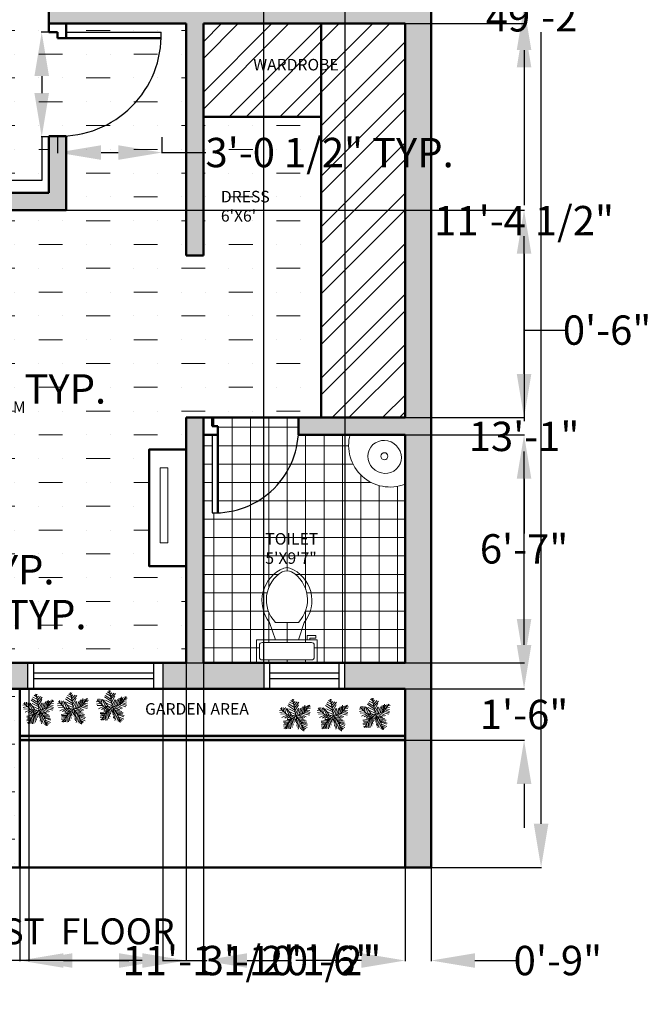
# Model space of a CAD drawing. Units: inches. Extents: x 26 to 14419, y 2 to 3479.
# Tile 7 of 9: x 14200 to 14419, y 2764 to 3106. Entities that reach past the tile are written whole.
import ezdxf

# ---------------------------------------------------------------- set-up
doc = ezdxf.new("R2010")
doc.units = ezdxf.units.IN
doc.header["$MEASUREMENT"] = 0
for name, color, linetype, lineweight in [('A-ANNO-DIMS', 2, 'Continuous', 18), ('A-ANNO-TEXT', 7, 'Continuous', 25), ('A-AREA-IDEN', 7, 'Continuous', 18), ('A-DOOR', 4, 'Continuous', 25), ('A-FLOR-FIXT', 8, 'Continuous', 18), ('A-FLOR-PATT', 252, 'Continuous', 13), ('A-GLAZ', 3, 'Continuous', 25), ('A-WALL', 7, 'Continuous', 50), ('L-PLNT', 3, 'Continuous', 13)]:
    doc.layers.add(name, color=color, linetype=linetype, lineweight=lineweight)
doc.styles.get("Standard").update_dxf_attribs({"font": 'arial.ttf'})
doc.dimstyles.get("Standard").update_dxf_attribs({"dimtxt": 10.18, "dimasz": 15.18, "dimexe": 0.18, "dimexo": 0.0625, "dimgap": 0.09, "dimtad": 0, "dimtih": 1, "dimtoh": 1, "dimdec": 0, "dimzin": 0, "dimdsep": 46, "dimlunit": 3, "dimtxsty": 'Standard', "dimcen": 0.09, "dimadec": 0, "dimazin": 0, "dimtfac": 1, "dimtdec": 0, "dimtofl": 0, "dimtmove": 0, "dimatfit": 3, "dimfxl": 1, "dimtolj": 1, "dimtzin": 0, "dimarcsym": 0})

# ---------------------------------------------------------------- blocks, each defined once
blk = doc.blocks.new('*U2')
for p, q in [((9.5, -6), (9.5, -2)), ((-10, -8.5), (-8, -8.5)), ((-10, -9.5), (-10, -8.5)), ((-7, -9.5), (-10, -9.5)), ((-8, -8.5), (-8, -8)), ((-7, -8), (-7, -9.5)), ((-4, -8), (-6, -14)), ((4, -8), (6, -14)), ((4, -14), (-4, -14))]:
    blk.add_line(p, q)
blk.add_lwpolyline([(10.5, -8), (10.5, 0), (-10.5, 0), (-10.5, -8)], close=True)
for points in [[(-9.5, -2), (-9.5, -6)], [(8.5, -1), (-8.5, -1)], [(-8.5, -7), (8.5, -7)]]:
    blk.add_lwpolyline(points)
for centre, radius, start, end in [((-8.62, -1.88), 0.884, 81.8699, 188.1301), ((8.62, -1.88), 0.884, 351.8699, 98.1301), ((-8.62, -6.12), 0.884, 171.8699, 278.1301), ((8.62, -6.12), 0.884, 261.8699, 8.1301), ((3.52, -21.58), 12.17, 141.4691, 247.9714), ((4.2, -21.82), 11.33, 136.3677, 238.9468), ((-3.52, -21.58), 12.17, 292.0284, 38.5307), ((-4.2, -21.82), 11.33, 301.053, 43.6321), ((0, -27.88), 4, 245.7318, 294.2682), ((0, -29), 4, 254.8605, 285.1395)]:
    blk.add_arc(centre, radius, start, end)
blk = doc.blocks.new('*U5')
for p, q in [((-3.665, 19.273), (-27.574, 35.527)), ((-5.114, 28.097), (-24.676, 40.636)), ((-7.288, 39.707), (-21.778, 46.673)), ((-8.737, 47.138), (-17.069, 52.711)), ((-10.186, 53.64), (-13.084, 55.962)), ((0, 0), (-10.5, 57)), ((-9.099, 51.782), (-6.563, 55.962)), ((-7.65, 43.423), (-2.578, 49.46)), ((-5.839, 35.992), (4.667, 48.067)), ((-5.114, 27.632), (10.463, 46.673)), ((-2.941, 16.486), (8.652, 37.85)), ((27, 9), (48, 36)), ((27.127, 9.056), (31.112, 35.992)), ((38.719, 34.134), (41.979, 28.561)), ((44.153, 36.456), (45.239, 32.741)), ((-47.498, 19.737), (-55.83, 18.344)), ((-40.615, 13.7), (-55.105, 10.913)), ((-31.5, 4.5), (-52.5, 25.5)), ((-33.37, 6.269), (-52.207, 5.34)), ((-48.585, 21.131), (-49.309, 29.026)), ((-28.299, 3.483), (-47.86, -5.805)), ((-43.513, 28.561), (-42.427, 15.558)), ((-38.442, 26.239), (-34.819, 7.663)), ((-21.416, 3.018), (-38.079, -8.128)), ((-35.544, 28.097), (-24.314, 3.947)), ((0, 0), (-31.5, 4.5)), ((-14.533, 2.09), (-30.834, 25.31)), ((-15.982, 2.09), (-30.11, -9.521)), ((-24.314, 23.917), (-2.941, 13.7)), ((0, 0), (-22.5, -19.5)), ((-6.563, 1.161), (-21.416, -8.128)), ((-20.691, 13.7), (-1.129, 4.876)), ((-1.129, 6.734), (9.014, 26.704)), ((0, 0), (27, 9)), ((0, 0), (18, -22.5)), ((3.942, 1.625), (11.187, 24.381)), ((6.478, 1.625), (26.04, -8.592)), ((10.101, 3.483), (17.708, 26.239)), ((11.187, 3.483), (30.749, -5.805)), ((16.259, 5.805), (23.142, 31.348)), ((18.07, 5.805), (35.096, -3.483)), ((22.055, 7.198), (27.489, 32.277)), ((24.229, 7.663), (46.688, 1.625)), ((29.662, 12.307), (48.137, 6.269)), ((31.836, 30.883), (32.561, 16.486)), ((33.285, 16.486), (48.862, 10.913)), ((35.096, 32.741), (37.27, 22.524)), ((36.183, 19.737), (48.137, 17.88)), ((40.53, 25.775), (48.862, 24.846)), ((43.791, 29.954), (51.036, 30.883)), ((-17.431, -15.094), (-42.789, -18.809)), ((-28.299, -29.026), (-42.789, -31.348)), ((-24.314, -21.596), (-42.427, -22.06)), ((-26.849, -26.24), (-40.253, -25.775)), ((-22.5, -19.5), (-37.5, -45)), ((-15.257, -12.772), (-30.11, -12.772)), ((-29.023, -30.884), (-27.936, -43.887)), ((-25.038, -23.918), (-22.865, -45.281)), ((-20.691, -18.345), (-17.793, -44.352)), ((-6.563, -5.805), (-19.967, -9.985)), ((-17.069, -15.094), (-12.721, -40.172)), ((-13.446, -11.378), (-8.737, -32.741)), ((-9.461, -8.592), (-6.201, -23.453)), ((-4.752, -3.483), (-3.665, -14.629)), ((2.493, -3.019), (-1.491, -20.202)), ((1.769, -2.555), (24.229, -9.521)), ((5.029, -6.27), (2.131, -25.775)), ((9.014, -11.378), (3.58, -35.992)), ((14.085, -16.951), (6.478, -40.172)), ((7.565, -9.056), (32.198, -14.629)), ((18.07, -22.524), (8.289, -45.745)), ((12.274, -15.094), (36.907, -18.809)), ((20.244, -30.419), (15.897, -44.816)), ((16.259, -19.738), (36.183, -22.989)), ((18, -22.5), (27, -52.5)), ((18.433, -22.524), (40.53, -29.026)), ((19.157, -25.311), (38.719, -33.206)), ((21.331, -32.741), (39.081, -40.636)), ((-30.834, -34.135), (-42.427, -35.528)), ((-34.457, -39.708), (-40.978, -42.494)), ((-32.646, -36.921), (-31.921, -44.352)), ((22.78, -37.85), (19.519, -48.532)), ((22.78, -38.314), (34.372, -44.816)), ((24.591, -45.745), (23.142, -50.854)), ((24.591, -43.423), (30.749, -47.603)), ((26.764, -49.925), (28.213, -50.854))]:
    blk.add_line(p, q)
blk = doc.blocks.new('*D9')
at = {"layer": 'A-ANNO-DIMS', "color": 0, "lineweight": -2, "transparency": 16777216}
for p, q in [((14342.71, 3401.72), (14380.97, 3401.72)), ((14380.79, 3386.54), (14380.79, 3112.01)), ((14380.79, 2826.9), (14380.79, 3101.43)), ((14342.71, 2811.72), (14380.97, 2811.72))]:
    blk.add_line(p, q, dxfattribs=at)
at = {"layer": 'A-ANNO-DIMS', "color": 0, "transparency": 16777216}
for points in [[(14378.26, 3386.54), (14383.32, 3386.54), (14380.79, 3401.72)], [(14378.26, 2826.9), (14383.32, 2826.9), (14380.79, 2811.72)]]:
    blk.add_solid(points, dxfattribs=at)
at = {"layer": 'Defpoints', "color": 0, "transparency": 16777216}
for p in [(14342.64, 3401.72), (14342.64, 2811.72), (14380.79, 2811.72)]:
    blk.add_point(p, dxfattribs=at)
at = {"layer": 'A-ANNO-DIMS', "color": 0, "transparency": 16777216, "insert": (14380.79, 3106.72), "char_height": 10.18, "attachment_point": 5}
blk.add_mtext('\\A1;49\'-2"', dxfattribs=at)
blk = doc.blocks.new('DOOR-900')
blk.add_line((0, 3), (0, 36))
blk.add_arc((1, 1), 35.01, 358.3634, 91.6366)
blk = doc.blocks.new('DOOR-750')
blk.add_line((3, 0), (30, 0))
blk.add_arc((1, 1), 29.02, 358.0251, 91.9749)
blk = doc.blocks.new('*D25')
at = {"layer": 'A-ANNO-DIMS', "color": 0, "lineweight": -2, "transparency": 16777216}
for p, q in [((14212.95, 3101.37), (14207.39, 3101.37)), ((14207.57, 3086.19), (14207.57, 3080.27)), ((14212.95, 3065.09), (14207.39, 3065.09)), ((14207.57, 3065.09), (14207.57, 3049.91)), ((14207.57, 3049.91), (14192.39, 3049.91))]:
    blk.add_line(p, q, dxfattribs=at)
at = {"layer": 'A-ANNO-DIMS', "color": 0, "transparency": 16777216}
for points in [[(14205.04, 3086.19), (14210.1, 3086.19), (14207.57, 3101.37)], [(14205.04, 3080.27), (14210.1, 3080.27), (14207.57, 3065.09)]]:
    blk.add_solid(points, dxfattribs=at)
at = {"layer": 'Defpoints', "color": 0, "transparency": 16777216}
for p in [(14213.01, 3101.37), (14207.57, 3065.09), (14213.01, 3065.09)]:
    blk.add_point(p, dxfattribs=at)
at = {"layer": 'A-ANNO-DIMS', "color": 0, "transparency": 16777216, "insert": (14112.52, 3049.91), "char_height": 10.18, "attachment_point": 5}
blk.add_mtext('\\A1;DOOR 900 3\'-0 1/2" TYP.', dxfattribs=at)
blk = doc.blocks.new('*D26')
at = {"layer": 'A-ANNO-DIMS', "color": 0, "lineweight": -2, "transparency": 16777216}
for p, q in [((14213.01, 3065.03), (14213.01, 3059.47)), ((14249.29, 3065.03), (14249.29, 3059.47)), ((14228.19, 3059.65), (14234.11, 3059.65)), ((14249.29, 3059.65), (14264.47, 3059.65))]:
    blk.add_line(p, q, dxfattribs=at)
at = {"layer": 'A-ANNO-DIMS', "color": 0, "transparency": 16777216}
for points in [[(14228.19, 3062.18), (14228.19, 3057.12), (14213.01, 3059.65)], [(14234.11, 3062.18), (14234.11, 3057.12), (14249.29, 3059.65)]]:
    blk.add_solid(points, dxfattribs=at)
at = {"layer": 'Defpoints', "color": 0, "transparency": 16777216}
for p in [(14213.01, 3065.09), (14249.29, 3065.09), (14249.29, 3059.65)]:
    blk.add_point(p, dxfattribs=at)
at = {"layer": 'A-ANNO-DIMS', "color": 0, "transparency": 16777216, "insert": (14307.44, 3059.65), "char_height": 10.18, "attachment_point": 5}
blk.add_mtext('\\A1;3\'-0 1/2" TYP.', dxfattribs=at)
blk = doc.blocks.new('*D39')
at = {"layer": 'A-ANNO-DIMS', "color": 0, "lineweight": -2, "transparency": 16777216}
for p, q in [((14110.79, 2942.13), (14110.79, 2957.31)), ((14107.27, 2926.95), (14110.97, 2926.95)), ((14107.27, 2903.04), (14110.97, 2903.04)), ((14110.79, 2887.86), (14110.79, 2872.68))]:
    blk.add_line(p, q, dxfattribs=at)
at = {"layer": 'A-ANNO-DIMS', "color": 0, "transparency": 16777216}
for points in [[(14108.26, 2942.13), (14113.32, 2942.13), (14110.79, 2926.95)], [(14108.26, 2887.86), (14113.32, 2887.86), (14110.79, 2903.04)]]:
    blk.add_solid(points, dxfattribs=at)
at = {"layer": 'Defpoints', "color": 0, "transparency": 16777216}
for p in [(14107.2, 2926.95), (14110.79, 2926.95), (14107.2, 2903.04)]:
    blk.add_point(p, dxfattribs=at)
at = {"layer": 'A-ANNO-DIMS', "color": 0, "transparency": 16777216, "insert": (14110.79, 2914.99), "char_height": 10.18, "attachment_point": 5}
blk.add_mtext('\\A1;SLATTED WARDROBE 2\'-0" TYP.', dxfattribs=at)
blk = doc.blocks.new('*D40')
at = {"layer": 'A-ANNO-DIMS', "color": 0, "lineweight": -2, "transparency": 16777216}
for p, q in [((14088.64, 2902.97), (14088.64, 2899.27)), ((14107.2, 2902.97), (14107.2, 2899.27)), ((14073.46, 2899.45), (14058.28, 2899.45)), ((14122.38, 2899.45), (14137.56, 2899.45))]:
    blk.add_line(p, q, dxfattribs=at)
at = {"layer": 'A-ANNO-DIMS', "color": 0, "transparency": 16777216}
for points in [[(14073.46, 2901.98), (14073.46, 2896.92), (14088.64, 2899.45)], [(14122.38, 2901.98), (14122.38, 2896.92), (14107.2, 2899.45)]]:
    blk.add_solid(points, dxfattribs=at)
at = {"layer": 'Defpoints', "color": 0, "transparency": 16777216}
for p in [(14088.64, 2903.04), (14107.2, 2903.04), (14107.2, 2899.45)]:
    blk.add_point(p, dxfattribs=at)
at = {"layer": 'A-ANNO-DIMS', "color": 0, "transparency": 16777216, "insert": (14180.06, 2899.45), "char_height": 10.18, "attachment_point": 5}
blk.add_mtext('\\A1;1\'-6 1/2" TYP.', dxfattribs=at)
blk = doc.blocks.new('*D44')
at = {"layer": 'A-ANNO-DIMS', "color": 0, "lineweight": -2, "transparency": 16777216}
for p, q in [((14079.96, 2977.68), (14064.78, 2977.68)), ((14095.14, 2980.15), (14095.14, 2977.5)), ((14105.73, 2980.15), (14105.73, 2977.5)), ((14120.91, 2977.68), (14136.09, 2977.68))]:
    blk.add_line(p, q, dxfattribs=at)
at = {"layer": 'A-ANNO-DIMS', "color": 0, "transparency": 16777216}
for points in [[(14079.96, 2980.21), (14079.96, 2975.15), (14095.14, 2977.68)], [(14120.91, 2980.21), (14120.91, 2975.15), (14105.73, 2977.68)]]:
    blk.add_solid(points, dxfattribs=at)
at = {"layer": 'Defpoints', "color": 0, "transparency": 16777216}
for p in [(14095.14, 2980.22), (14105.73, 2980.22), (14105.73, 2977.68)]:
    blk.add_point(p, dxfattribs=at)
at = {"layer": 'A-ANNO-DIMS', "color": 0, "transparency": 16777216, "insert": (14183.02, 2977.68), "char_height": 10.18, "attachment_point": 5}
blk.add_mtext('\\A1;0\'-10 1/2" TYP.', dxfattribs=at)
blk = doc.blocks.new('*D86')
at = {"layer": 'A-ANNO-DIMS', "color": 0, "lineweight": -2, "transparency": 16777216}
for p, q in [((14199.93, 2811.66), (14199.93, 2779.29)), ((14333.64, 2811.66), (14333.64, 2779.29)), ((14215.11, 2779.47), (14237.83, 2779.47)), ((14318.46, 2779.47), (14295.74, 2779.47))]:
    blk.add_line(p, q, dxfattribs=at)
at = {"layer": 'A-ANNO-DIMS', "color": 0, "transparency": 16777216}
for points in [[(14215.11, 2782), (14215.11, 2776.94), (14199.93, 2779.47)], [(14318.46, 2782), (14318.46, 2776.94), (14333.64, 2779.47)]]:
    blk.add_solid(points, dxfattribs=at)
at = {"layer": 'Defpoints', "color": 0, "transparency": 16777216}
for p in [(14199.93, 2811.72), (14333.64, 2811.72), (14333.64, 2779.47)]:
    blk.add_point(p, dxfattribs=at)
at = {"layer": 'A-ANNO-DIMS', "color": 0, "transparency": 16777216, "insert": (14266.78, 2779.47), "char_height": 10.18, "attachment_point": 5}
blk.add_mtext('\\A1;11\'-1 1/2"', dxfattribs=at)
blk = doc.blocks.new('*D87')
at = {"layer": 'A-ANNO-DIMS', "color": 0, "lineweight": -2, "transparency": 16777216}
for p, q in [((14333.64, 2811.66), (14333.64, 2779.29)), ((14342.64, 2811.66), (14342.64, 2779.29)), ((14318.46, 2779.47), (14303.28, 2779.47)), ((14357.82, 2779.47), (14373, 2779.47))]:
    blk.add_line(p, q, dxfattribs=at)
at = {"layer": 'A-ANNO-DIMS', "color": 0, "transparency": 16777216}
for points in [[(14318.46, 2782), (14318.46, 2776.94), (14333.64, 2779.47)], [(14357.82, 2782), (14357.82, 2776.94), (14342.64, 2779.47)]]:
    blk.add_solid(points, dxfattribs=at)
at = {"layer": 'Defpoints', "color": 0, "transparency": 16777216}
for p in [(14333.64, 2811.72), (14342.64, 2811.72), (14342.64, 2779.47)]:
    blk.add_point(p, dxfattribs=at)
at = {"layer": 'A-ANNO-DIMS', "color": 0, "transparency": 16777216, "insert": (14386.62, 2779.47), "char_height": 10.18, "attachment_point": 5}
blk.add_mtext('\\A1;0\'-9"', dxfattribs=at)
blk = doc.blocks.new('*D90')
at = {"layer": 'A-ANNO-DIMS', "color": 0, "lineweight": -2, "transparency": 16777216}
for p, q in [((14216.08, 3039.72), (14375.07, 3039.72)), ((14374.89, 3024.54), (14374.89, 2966.51)), ((14374.89, 2897.9), (14374.89, 2955.93)), ((14257.71, 2882.72), (14375.07, 2882.72))]:
    blk.add_line(p, q, dxfattribs=at)
at = {"layer": 'A-ANNO-DIMS', "color": 0, "transparency": 16777216}
for points in [[(14372.36, 3024.54), (14377.42, 3024.54), (14374.89, 3039.72)], [(14372.36, 2897.9), (14377.42, 2897.9), (14374.89, 2882.72)]]:
    blk.add_solid(points, dxfattribs=at)
at = {"layer": 'Defpoints', "color": 0, "transparency": 16777216}
for p in [(14216.01, 3039.72), (14257.64, 2882.72), (14374.89, 2882.72)]:
    blk.add_point(p, dxfattribs=at)
at = {"layer": 'A-ANNO-DIMS', "color": 0, "transparency": 16777216, "insert": (14374.89, 2961.22), "char_height": 10.18, "attachment_point": 5}
blk.add_mtext('\\A1;13\'-1"', dxfattribs=at)
blk = doc.blocks.new('*D99')
at = {"layer": 'A-ANNO-DIMS', "color": 0, "lineweight": -2, "transparency": 16777216}
for p, q in [((14374.89, 2888.9), (14374.89, 2904.08)), ((14333.71, 2873.72), (14375.07, 2873.72)), ((14333.71, 2855.88), (14375.07, 2855.88)), ((14374.89, 2840.7), (14374.89, 2825.52))]:
    blk.add_line(p, q, dxfattribs=at)
at = {"layer": 'A-ANNO-DIMS', "color": 0, "transparency": 16777216}
for points in [[(14372.36, 2888.9), (14377.42, 2888.9), (14374.89, 2873.72)], [(14372.36, 2840.7), (14377.42, 2840.7), (14374.89, 2855.88)]]:
    blk.add_solid(points, dxfattribs=at)
at = {"layer": 'Defpoints', "color": 0, "transparency": 16777216}
for p in [(14333.64, 2873.72), (14374.89, 2873.72), (14333.64, 2855.88)]:
    blk.add_point(p, dxfattribs=at)
at = {"layer": 'A-ANNO-DIMS', "color": 0, "transparency": 16777216, "insert": (14374.89, 2864.8), "char_height": 10.18, "attachment_point": 5}
blk.add_mtext('\\A1;1\'-6"', dxfattribs=at)
blk = doc.blocks.new('*D100')
at = {"layer": 'A-ANNO-DIMS', "color": 0, "lineweight": -2, "transparency": 16777216}
for p, q in [((14333.71, 2961.72), (14375.07, 2961.72)), ((14374.89, 2946.54), (14374.89, 2927.51)), ((14374.89, 2897.9), (14374.89, 2916.93)), ((14333.71, 2882.72), (14375.07, 2882.72))]:
    blk.add_line(p, q, dxfattribs=at)
at = {"layer": 'A-ANNO-DIMS', "color": 0, "transparency": 16777216}
for points in [[(14372.36, 2946.54), (14377.42, 2946.54), (14374.89, 2961.72)], [(14372.36, 2897.9), (14377.42, 2897.9), (14374.89, 2882.72)]]:
    blk.add_solid(points, dxfattribs=at)
at = {"layer": 'Defpoints', "color": 0, "transparency": 16777216}
for p in [(14333.64, 2961.72), (14374.89, 2961.72), (14333.64, 2882.72)]:
    blk.add_point(p, dxfattribs=at)
at = {"layer": 'A-ANNO-DIMS', "color": 0, "transparency": 16777216, "insert": (14374.89, 2922.22), "char_height": 10.18, "attachment_point": 5}
blk.add_mtext('\\A1;6\'-7"', dxfattribs=at)
blk = doc.blocks.new('*D101')
at = {"layer": 'A-ANNO-DIMS', "color": 0, "lineweight": -2, "transparency": 16777216}
for p, q in [((14374.89, 2982.9), (14374.89, 2998.08)), ((14374.89, 2998.08), (14390.07, 2998.08)), ((14333.71, 2967.72), (14375.07, 2967.72)), ((14333.71, 2961.72), (14375.07, 2961.72)), ((14374.89, 2946.54), (14374.89, 2931.36))]:
    blk.add_line(p, q, dxfattribs=at)
at = {"layer": 'A-ANNO-DIMS', "color": 0, "transparency": 16777216}
for points in [[(14372.36, 2982.9), (14377.42, 2982.9), (14374.89, 2967.72)], [(14372.36, 2946.54), (14377.42, 2946.54), (14374.89, 2961.72)]]:
    blk.add_solid(points, dxfattribs=at)
at = {"layer": 'Defpoints', "color": 0, "transparency": 16777216}
for p in [(14333.64, 2967.72), (14374.89, 2967.72), (14333.64, 2961.72)]:
    blk.add_point(p, dxfattribs=at)
at = {"layer": 'A-ANNO-DIMS', "color": 0, "transparency": 16777216, "insert": (14403.69, 2998.08), "char_height": 10.18, "attachment_point": 5}
blk.add_mtext('\\A1;0\'-6"', dxfattribs=at)
blk = doc.blocks.new('*D102')
at = {"layer": 'A-ANNO-DIMS', "color": 0, "lineweight": -2, "transparency": 16777216}
for p, q in [((14333.71, 3104.37), (14375.07, 3104.37)), ((14374.89, 3089.19), (14374.89, 3041.4)), ((14374.89, 2982.9), (14374.89, 3030.69)), ((14333.71, 2967.72), (14375.07, 2967.72))]:
    blk.add_line(p, q, dxfattribs=at)
at = {"layer": 'A-ANNO-DIMS', "color": 0, "transparency": 16777216}
for points in [[(14372.36, 3089.19), (14377.42, 3089.19), (14374.89, 3104.37)], [(14372.36, 2982.9), (14377.42, 2982.9), (14374.89, 2967.72)]]:
    blk.add_solid(points, dxfattribs=at)
at = {"layer": 'Defpoints', "color": 0, "transparency": 16777216}
for p in [(14333.64, 3104.37), (14374.89, 3104.37), (14333.64, 2967.72)]:
    blk.add_point(p, dxfattribs=at)
at = {"layer": 'A-ANNO-DIMS', "color": 0, "transparency": 16777216, "insert": (14374.89, 3036.04), "char_height": 10.18, "attachment_point": 5}
blk.add_mtext('\\A1;11\'-4 1/2"', dxfattribs=at)
blk = doc.blocks.new('*D110')
at = {"layer": 'A-ANNO-DIMS', "color": 0, "lineweight": -2, "transparency": 16777216}
for p, q in [((14088.64, 2882.66), (14088.64, 2779.29)), ((14257.64, 2882.66), (14257.64, 2779.29)), ((14103.82, 2779.47), (14156.05, 2779.47)), ((14242.46, 2779.47), (14190.24, 2779.47))]:
    blk.add_line(p, q, dxfattribs=at)
at = {"layer": 'A-ANNO-DIMS', "color": 0, "transparency": 16777216}
for points in [[(14103.82, 2782), (14103.82, 2776.94), (14088.64, 2779.47)], [(14242.46, 2782), (14242.46, 2776.94), (14257.64, 2779.47)]]:
    blk.add_solid(points, dxfattribs=at)
at = {"layer": 'Defpoints', "color": 0, "transparency": 16777216}
for p in [(14088.64, 2882.72), (14257.64, 2882.72), (14257.64, 2779.47)]:
    blk.add_point(p, dxfattribs=at)
at = {"layer": 'A-ANNO-DIMS', "color": 0, "transparency": 16777216, "insert": (14173.14, 2779.47), "char_height": 10.18, "attachment_point": 5}
blk.add_mtext('\\A1;14\'-1"', dxfattribs=at)
blk = doc.blocks.new('*D111')
at = {"layer": 'A-ANNO-DIMS', "color": 0, "lineweight": -2, "transparency": 16777216}
for p, q in [((14257.64, 2967.66), (14257.64, 2779.29)), ((14263.64, 2967.66), (14263.64, 2779.29)), ((14242.46, 2779.47), (14227.28, 2779.47)), ((14278.82, 2779.47), (14294, 2779.47))]:
    blk.add_line(p, q, dxfattribs=at)
at = {"layer": 'A-ANNO-DIMS', "color": 0, "transparency": 16777216}
for points in [[(14242.46, 2782), (14242.46, 2776.94), (14257.64, 2779.47)], [(14278.82, 2782), (14278.82, 2776.94), (14263.64, 2779.47)]]:
    blk.add_solid(points, dxfattribs=at)
at = {"layer": 'Defpoints', "color": 0, "transparency": 16777216}
for p in [(14257.64, 2967.72), (14263.64, 2967.72), (14263.64, 2779.47)]:
    blk.add_point(p, dxfattribs=at)
at = {"layer": 'A-ANNO-DIMS', "color": 0, "transparency": 16777216, "insert": (14307.62, 2779.47), "char_height": 10.18, "attachment_point": 5}
blk.add_mtext('\\A1;0\'-6"', dxfattribs=at)
blk = doc.blocks.new('*D112')
at = {"layer": 'A-ANNO-DIMS', "color": 0, "lineweight": -2, "transparency": 16777216}
for p, q in [((14269.46, 3433.97), (14254.28, 3433.97)), ((14284.64, 2882.78), (14284.64, 3434.15)), ((14312.82, 2882.82), (14312.82, 3434.15)), ((14328, 3433.97), (14343.18, 3433.97))]:
    blk.add_line(p, q, dxfattribs=at)
at = {"layer": 'A-ANNO-DIMS', "color": 0, "transparency": 16777216}
for points in [[(14269.46, 3436.5), (14269.46, 3431.44), (14284.64, 3433.97)], [(14328, 3436.5), (14328, 3431.44), (14312.82, 3433.97)]]:
    blk.add_solid(points, dxfattribs=at)
at = {"layer": 'Defpoints', "color": 0, "transparency": 16777216}
for p in [(14312.82, 3433.97), (14284.64, 2882.72), (14312.82, 2882.76)]:
    blk.add_point(p, dxfattribs=at)
at = {"layer": 'A-ANNO-DIMS', "color": 0, "transparency": 16777216, "insert": (14298.73, 3433.97), "char_height": 10.18, "attachment_point": 5}
blk.add_mtext('\\A1;2\'-4"', dxfattribs=at)
blk = doc.blocks.new('*D116')
at = {"layer": 'A-ANNO-DIMS', "color": 0, "lineweight": -2, "transparency": 16777216}
for p, q in [((14203.05, 2873.83), (14203.05, 2779.29)), ((14249.61, 2873.66), (14249.61, 2779.29)), ((14218.23, 2779.47), (14234.43, 2779.47)), ((14249.61, 2779.47), (14264.79, 2779.47))]:
    blk.add_line(p, q, dxfattribs=at)
at = {"layer": 'A-ANNO-DIMS', "color": 0, "transparency": 16777216}
for points in [[(14218.23, 2782), (14218.23, 2776.94), (14203.05, 2779.47)], [(14234.43, 2782), (14234.43, 2776.94), (14249.61, 2779.47)]]:
    blk.add_solid(points, dxfattribs=at)
at = {"layer": 'Defpoints', "color": 0, "transparency": 16777216}
for p in [(14203.05, 2873.89), (14249.61, 2873.72), (14249.61, 2779.47)]:
    blk.add_point(p, dxfattribs=at)
at = {"layer": 'A-ANNO-DIMS', "color": 0, "transparency": 16777216, "insert": (14294.23, 2779.47), "char_height": 10.18, "attachment_point": 5}
blk.add_mtext('\\A1;3\'-10 1/2"', dxfattribs=at)
blk = doc.blocks.new('*D119')
at = {"layer": 'A-ANNO-DIMS', "color": 0, "lineweight": -2, "transparency": 16777216}
for p, q in [((14374.89, 3152.72), (14374.89, 3167.9)), ((14297.71, 3137.54), (14375.07, 3137.54)), ((14297.71, 3110.37), (14375.07, 3110.37)), ((14374.89, 3095.19), (14374.89, 3080.01))]:
    blk.add_line(p, q, dxfattribs=at)
at = {"layer": 'A-ANNO-DIMS', "color": 0, "transparency": 16777216}
for points in [[(14372.36, 3152.72), (14377.42, 3152.72), (14374.89, 3137.54)], [(14372.36, 3095.19), (14377.42, 3095.19), (14374.89, 3110.37)]]:
    blk.add_solid(points, dxfattribs=at)
at = {"layer": 'Defpoints', "color": 0, "transparency": 16777216}
for p in [(14297.64, 3137.54), (14374.89, 3137.54), (14297.64, 3110.37)]:
    blk.add_point(p, dxfattribs=at)
at = {"layer": 'A-ANNO-DIMS', "color": 0, "transparency": 16777216, "insert": (14374.89, 3123.96), "char_height": 10.18, "attachment_point": 5}
blk.add_mtext('\\A1;2\'-3"', dxfattribs=at)

msp = doc.modelspace()

# ---------------------------------------------------------------- hatches: boundary and pattern name
at = {"layer": 'A-FLOR-PATT'}
h = msp.add_hatch(color=256, dxfattribs=at)
h.dxf.hatch_style = 1
h.paths.add_polyline_path([(13922.09, 3432), (13659.09, 3432), (13659.09, 2842), (13668.09, 2842), (13668.09, 2851), (13668.09, 2899), (13668.09, 2908), (13668.09, 3076), (13706.09, 3076), (13706.09, 3085), (13668.09, 3085), (13668.09, 3249), (13712.76, 3249), (13712.76, 3255), (13668.09, 3255), (13668.09, 3375), (13720.94, 3375), (13720.94, 3378, -0.017236), (13720.94, 3380), (13720.94, 3381), (13668.09, 3381), (13668.09, 3423), (13784.09, 3423), (13784.09, 3381), (13753.94, 3381), (13753.94, 3375), (13784.09, 3375), (13784.09, 3255), (13758.77, 3255), (13758.77, 3249), (13784.09, 3249), (13793.09, 3249), (13793.09, 3255), (13793.09, 3423), (13913.09, 3423), (13913.09, 3255), (13832.09, 3255), (13832.09, 3254, -0.014283), (13832.09, 3252), (13832.09, 3249), (13836.57, 3249), (13836.57, 3234), (13839.57, 3234, -0.017236), (13841.57, 3234), (13842.57, 3234), (13842.57, 3249), (13913.09, 3249), (13913.09, 3201), (13892.46, 3201), (13793.09, 3201), (13784.09, 3201), (13784.09, 3195), (13793.09, 3195), (13913.09, 3195), (13913.09, 3127), (13922.09, 3127)])
h.paths.add_polyline_path([(13922.09, 3013.5), (13913.09, 3013.5), (13913.09, 2908), (13892.09, 2908), (13892.09, 2899), (13913.09, 2899), (13913.09, 2851), (13793.09, 2851), (13784.09, 2851), (13784.09, 2842), (13922.09, 2842)], flags=17)
h.paths.add_polyline_path([(13793.09, 3085), (13784.09, 3085), (13784.09, 3076), (13784.09, 3071.08), (13784.09, 3066.17), (13784.09, 2908), (13784.09, 2899.07), (13793.09, 2899), (13802.09, 2899), (13814.09, 2899), (13814.09, 2908), (13793.09, 2908)], flags=17)
h.paths.add_polyline_path([(14342.64, 3401.72), (14242.78, 3401.72), (14242.78, 3392.72), (14257.64, 3392.72), (14257.64, 3351.75), (14257.64, 3345.75), (14257.64, 3330.73), (14263.64, 3330.73), (14263.64, 3392.72), (14333.64, 3392.72), (14333.64, 3284.72), (14302.92, 3284.72), (14302.92, 3281.72, -0.022645), (14302.92, 3279.12), (14302.92, 3278.72), (14333.64, 3278.72), (14333.64, 3170.72), (14316.1, 3170.72), (14263.64, 3170.72), (14263.64, 3278.72), (14269.92, 3278.72), (14269.92, 3284.72), (14263.64, 3284.72), (14257.64, 3284.72), (14257.64, 3225.75), (14257.64, 3219.75), (14257.64, 3164.72), (14333.64, 3164.72), (14333.64, 3110.37), (14210.01, 3110.37), (14210.01, 3104.37), (14257.64, 3104.37), (14257.64, 3024), (14263.64, 3024), (14263.64, 3039.72), (14263.64, 3104.37), (14333.64, 3104.37), (14333.64, 3045.72), (14333.64, 3039.72), (14333.64, 2967.72), (14296.64, 2967.72), (14296.64, 2964.72, -0.017236), (14296.64, 2962.72), (14296.64, 2961.72), (14333.64, 2961.72), (14333.64, 2882.72), (14312.64, 2882.72), (14312.64, 2873.72), (14333.64, 2873.72), (14333.64, 2820.72), (14333.64, 2811.72), (14342.64, 2811.72)])
h.paths.add_polyline_path([(14088.64, 3219.75), (14218.64, 3219.75), (14218.64, 3222.75, -0.014283), (14218.64, 3224.75), (14218.64, 3225.75), (14088.64, 3225.75), (14088.64, 3345.75), (14088.64, 3351.75), (14088.64, 3392.72), (14193.93, 3392.72), (14193.93, 3351.75), (14140.64, 3351.75), (14140.64, 3345.75), (14170.7, 3345.75), (14218.64, 3345.75), (14218.64, 3348.75, -0.014283), (14218.64, 3350.75), (14218.64, 3351.75), (14199.93, 3351.75), (14199.93, 3392.72), (14214.78, 3392.72), (14214.78, 3401.72), (14079.64, 3401.72), (14079.64, 2811.72), (14088.64, 2811.72), (14088.64, 2820.72), (14088.64, 2873.72), (14116.21, 2873.72), (14116.21, 2876.57), (14116.21, 2882.72), (14088.64, 2882.72), (14088.64, 3039.72), (14216.01, 3039.72), (14216.01, 3065.37), (14215.01, 3065.37, -0.014283), (14213.01, 3065.37), (14210.01, 3065.37), (14210.01, 3045.72), (14154.64, 3045.72), (14148.64, 3045.72), (14088.64, 3045.72)])
h.paths.add_polyline_path([(14284.64, 2882.72), (14263.64, 2882.72), (14263.64, 2961.72), (14263.64, 2967.72), (14257.64, 2967.72), (14257.64, 2956.69), (14257.64, 2916.18), (14257.64, 2882.72), (14249.61, 2882.72), (14249.61, 2873.72), (14284.64, 2873.72)], flags=17)
h.paths.add_polyline_path([(14202.78, 2882.72), (14189.55, 2882.72), (14189.55, 2879.95), (14189.55, 2873.72), (14202.78, 2873.72)], flags=17)
h = msp.add_hatch(dxfattribs=at)
h.set_pattern_fill('MUDST', color=256, scale=33)
h.paths.add_polyline_path([(14304.4, 3368.55), (14263.64, 3368.55), (14263.64, 3330.73), (14257.64, 3330.73), (14257.64, 3345.75), (14254.64, 3345.75), (14254.64, 3348.75), (14252.64, 3348.75), (14252.64, 3384.75, 0.397579), (14218.64, 3350.75), (14218.64, 3345.75), (14170.7, 3345.75), (14170.7, 3274.26), (14114.64, 3274.26), (14114.64, 3345.75), (14088.64, 3345.75), (14088.64, 3225.75), (14114.67, 3225.75), (14114.67, 3239.54), (14174.56, 3239.54), (14174.56, 3225.75), (14218.69, 3225.75, -0.405865), (14254.64, 3258.75), (14254.64, 3225.75), (14257.64, 3225.75), (14257.64, 3284.72), (14263.64, 3284.72), (14272.92, 3284.72), (14272.92, 3281.72), (14274.92, 3281.72), (14274.92, 3251.72, 0.394163), (14302.92, 3279.12), (14302.92, 3284.72), (14304.4, 3284.72)])
h.paths.add_polyline_path([(14189.03, 3330.51), (14176.21, 3330.51), (14176.21, 3342.77), (14189.03, 3342.77)], flags=16)
h.paths.add_polyline_path([(14188.03, 3331.51), (14177.21, 3331.51), (14177.21, 3341.77), (14188.03, 3341.77)], flags=0)
h.paths.add_polyline_path([(14185.02, 3336.64, -1), (14180.21, 3336.64, -1)], flags=0)
h.paths.add_polyline_path([(14109.33, 3330.51), (14096.5, 3330.51), (14096.5, 3342.77), (14109.33, 3342.77)], flags=16)
h.paths.add_polyline_path([(14108.33, 3331.51), (14097.5, 3331.51), (14097.5, 3341.77), (14108.33, 3341.77)], flags=0)
h.paths.add_polyline_path([(14105.32, 3336.64, -1), (14100.51, 3336.64, -1)], flags=0)
h.paths.add_polyline_path([(14257.64, 3219.75), (14254.64, 3219.75), (14254.64, 3222.75), (14252.64, 3222.75), (14252.64, 3258.75, 0.397579), (14218.64, 3224.75), (14218.64, 3219.75), (14088.64, 3219.75), (14088.64, 3105.72), (14154.64, 3105.72), (14154.64, 3045.72), (14210.01, 3045.72), (14210.01, 3065.37), (14215.01, 3065.37, 0.397579), (14249.01, 3099.37), (14213.01, 3099.37), (14213.01, 3101.37), (14210.01, 3101.37), (14210.01, 3110.37), (14217.64, 3110.37), (14217.64, 3164.72), (14215.11, 3164.72), (14215.11, 3170.72), (14257.64, 3170.72)])
h.paths.add_polyline_path([(14174.2, 3192.28), (14172.21, 3192.28), (14172.21, 3190.47), (14113.94, 3190.47), (14113.94, 3192.28), (14112.02, 3192.28), (14112.02, 3207.65), (14113.94, 3207.65), (14174.2, 3207.65)], flags=16)
h.paths.add_polyline_path([(14132.26, 3203.31), (14132.26, 3205.54), (14153.01, 3205.54), (14153.01, 3203.31)], flags=0)
h.paths.add_polyline_path([(14139.45, 3178.77), (14139.45, 3144.03), (14124.04, 3144.03), (14124.04, 3178.77)], flags=16)
h.paths.add_polyline_path([(14138.45, 3177.77), (14138.45, 3145.03), (14125.04, 3145.03), (14125.04, 3177.77)], flags=0)
h.paths.add_polyline_path([(14127.62, 3154.26), (14127.69, 3154.32), (14127.65, 3154.8), (14127.17, 3154.71)], flags=0)
h.paths.add_polyline_path([(14137.62, 3155.43), (14138.07, 3155.38), (14137.86, 3155.74)], flags=0)
h.paths.add_polyline_path([(14134.11, 3152.76), (14134.62, 3152.52), (14134.75, 3152.98)], flags=0)
h.paths.add_polyline_path([(14134.97, 3149.61), (14135.06, 3149.3), (14135.3, 3149.21), (14134.97, 3149.61)], flags=0)
h.paths.add_polyline_path([(14129.06, 3148.22), (14128.85, 3148.19), (14128.88, 3147.91)], flags=0)
h.paths.add_polyline_path([(14129.76, 3149.73), (14129.77, 3149.7), (14129.81, 3149.73)], flags=0)
h.paths.add_polyline_path([(14129.81, 3152.94), (14129.51, 3152.8), (14129.91, 3152.74)], flags=0)
h.paths.add_polyline_path([(14129.97, 3154.13), (14131.4, 3152.09), (14132.47, 3152.75), (14132.58, 3152.96)], flags=0)
h.paths.add_polyline_path([(14131.76, 3158.63), (14131.62, 3158.74), (14131.67, 3158.49)], flags=0)
h.paths.add_polyline_path([(14133.11, 3151.99), (14133.11, 3152.01), (14133.11, 3151.99)], flags=0)
h.paths.add_polyline_path([(14135.18, 3148.48), (14135.04, 3148), (14135.53, 3147.73), (14135.69, 3148.25)], flags=0)
h.paths.add_polyline_path([(14111.74, 3127.44), (14109.92, 3127.44), (14109.92, 3125.52), (14094.56, 3125.52), (14094.56, 3127.44), (14094.56, 3187.7), (14109.92, 3187.7), (14109.92, 3185.71), (14111.74, 3185.71)], flags=16)
h.paths.add_polyline_path([(14098.89, 3166.51), (14098.89, 3145.76), (14096.67, 3145.76), (14096.67, 3166.51)], flags=0)
h.paths.add_polyline_path([(14107.98, 3191.64), (14092.66, 3191.64), (14092.66, 3205.45), (14107.98, 3205.45)], flags=16)
h.paths.add_polyline_path([(14102.61, 3192.64), (14102.72, 3192.57), (14102.74, 3192.64)], flags=0)
h.paths.add_polyline_path([(14101.15, 3198.79), (14101.66, 3198.55), (14101.79, 3199)], flags=0)
h.paths.add_polyline_path([(14105.37, 3201.99), (14105.29, 3202.26), (14105.04, 3201.95)], flags=0)
h.paths.add_polyline_path([(14102.01, 3195.63), (14102.11, 3195.33), (14102.34, 3195.23), (14102.02, 3195.64)], flags=0)
h.paths.add_polyline_path([(14102.22, 3194.5), (14102.08, 3194.03), (14102.57, 3193.75), (14102.73, 3194.27)], flags=0)
h.paths.add_polyline_path([(14096.1, 3194.24), (14095.89, 3194.22), (14095.92, 3193.93)], flags=0)
h.paths.add_polyline_path([(14096.81, 3195.75), (14096.81, 3195.72), (14096.85, 3195.75)], flags=0)
h.paths.add_polyline_path([(14094.74, 3200.21), (14094.69, 3200.82), (14094.21, 3200.74)], flags=0)
h.paths.add_polyline_path([(14096.86, 3198.97), (14096.55, 3198.82), (14096.95, 3198.77)], flags=0)
h.paths.add_polyline_path([(14097.01, 3200.16), (14098.44, 3198.11), (14099.51, 3198.78), (14099.62, 3198.98)], flags=0)
h.paths.add_polyline_path([(14098.8, 3204.66), (14098.66, 3204.77), (14098.71, 3204.51)], flags=0)
h.paths.add_polyline_path([(14100.15, 3198.02), (14100.15, 3198.03), (14100.15, 3198.02)], flags=0)
h.paths.add_polyline_path([(14257.64, 2967.72), (14263.64, 2967.72), (14266.64, 2967.72), (14296.64, 2967.72), (14304.52, 2967.72), (14304.52, 3072.04), (14263.64, 3072.04), (14263.64, 3039.72), (14263.64, 3024), (14257.64, 3024), (14257.64, 3104.37), (14216.01, 3104.37), (14216.01, 3101.37), (14249.01, 3101.37, -0.405865), (14216.01, 3065.41), (14216.01, 3039.72), (14088.64, 3039.72), (14088.64, 3034.24), (14107.2, 3034.24), (14107.2, 3010.33), (14088.64, 3010.33), (14088.64, 3001.38), (14176.64, 3001.38), (14176.64, 2931.05), (14088.64, 2931.05), (14088.64, 2926.95), (14107.2, 2926.95), (14107.2, 2903.04), (14088.64, 2903.04), (14088.64, 2882.72), (14116.21, 2882.72), (14116.21, 2876.57), (14151.84, 2876.57), (14151.84, 2882.72), (14189.55, 2882.72), (14257.64, 2882.72), (14257.64, 2916.18), (14244.9, 2916.18), (14244.9, 2956.69), (14257.64, 2956.69)])
h.paths.add_polyline_path([(14199.2, 2873.72), (14189.55, 2873.72), (14189.55, 2879.95), (14151.84, 2879.95), (14151.84, 2873.72), (14116.21, 2873.72), (14088.64, 2873.72), (14088.64, 2820.72), (14088.64, 2813.09), (14199.2, 2813.09)])
h.paths.add_polyline_path([(14272.13, 3336.81), (14293.39, 3336.81), (14293.39, 3351.73), (14272.13, 3351.73)], flags=24)
h.paths.add_polyline_path([(14208.53, 3375.98), (14237.24, 3375.98), (14237.24, 3384.22), (14208.53, 3384.22)], flags=25)
h.paths.add_polyline_path([(14136.68, 3250.57), (14220.54, 3250.57), (14220.54, 3272.96), (14136.68, 3272.96)], flags=24)
h.paths.add_polyline_path([(14121.4, 3116.81), (14182.4, 3116.81), (14182.4, 3131.73), (14121.4, 3131.73)], flags=24)
h.paths.add_polyline_path([(14268.29, 3033.43), (14289.54, 3033.43), (14289.54, 3048.36), (14268.29, 3048.36)], flags=24)
h.paths.add_polyline_path([(14151.68, 2960.42), (14207.58, 2960.42), (14207.58, 2975.35), (14151.68, 2975.35)], flags=25)
h.paths.add_polyline_path([(14128.74, 2839.15), (14157.44, 2839.15), (14157.44, 2847.39), (14128.74, 2847.39)], flags=24)
h = msp.add_hatch(dxfattribs=at)
h.set_pattern_fill('ANSI32', color=256, scale=33)
h.paths.add_polyline_path([(14304.52, 3104.37), (14263.64, 3104.37), (14263.64, 3072.04), (14304.52, 3072.04)])
h.paths.add_polyline_path([(14333.64, 3104.37), (14304.52, 3104.37), (14304.52, 3072.04), (14304.52, 2967.72), (14333.64, 2967.72), (14333.64, 3039.72), (14333.64, 3045.72)])
h = msp.add_hatch(dxfattribs=at)
h.set_pattern_fill('NET', color=256, scale=51)
h.paths.add_polyline_path([(14333.64, 2944.65, -0.612791), (14314.5, 2961.72), (14296.59, 2961.72, -0.404142), (14266.64, 2934.72), (14266.64, 2961.72), (14263.64, 2961.72), (14263.64, 2882.72), (14333.64, 2882.72)])
h.paths.add_polyline_path([(14294.28, 2914.24, -0.48008), (14296.63, 2896.72), (14288.63, 2896.72, -0.48008), (14290.99, 2914.24, -0.215004)], flags=16)
h.paths.add_polyline_path([(14301.13, 2889.72, -0.5), (14302.13, 2888.72), (14302.13, 2884.72, -0.5), (14301.13, 2883.72), (14284.13, 2883.72, -0.5), (14283.13, 2884.72), (14283.13, 2888.72, -0.5), (14284.13, 2889.72)], flags=16)
h.paths.add_polyline_path([(14296.59, 2961.72, 0.008628), (14296.64, 2962.72), (14296.64, 2967.72), (14266.64, 2967.72), (14266.64, 2964.72), (14268.64, 2964.72), (14268.64, 2934.72, 0.384229)])
h = msp.add_hatch(color=256, dxfattribs=at)
h.dxf.hatch_style = 1
h.paths.add_polyline_path([(14333.64, 2857.41), (14199.93, 2857.41), (14199.93, 2855.88), (14333.64, 2855.88)])

# ---------------------------------------------------------------- linework, layer by layer
at = {"layer": 'A-FLOR-FIXT'}
msp.add_lwpolyline([(14251.27, 2950.35), (14248.64, 2950.35), (14248.64, 2924.26), (14251.27, 2924.26)], close=True, dxfattribs=at)
msp.add_circle((14326.45, 2954.34), 1.22, dxfattribs=at)
msp.add_arc((14328.42, 2958.06), 14.39, 164.4013, 291.0805, dxfattribs=at)
at = {"layer": 'A-FLOR-FIXT', "extrusion": (0, 0, -1)}
msp.add_ellipse((14326.52, 2954.11), major_axis=(-4.81, 3.38), ratio=0.960909, start_param=-6.283185, end_param=0, dxfattribs=at)
at = {"layer": 'A-GLAZ'}
for p, q in [((14202.78, 2873.72), (14202.78, 2882.72)), ((14204.74, 2882.72), (14204.74, 2873.72)), ((14246.35, 2882.72), (14246.35, 2873.72)), ((14249.61, 2882.72), (14249.61, 2873.72)), ((14284.64, 2882.72), (14284.64, 2873.72)), ((14286.64, 2882.72), (14286.64, 2873.72)), ((14310.64, 2882.72), (14310.64, 2873.72)), ((14312.64, 2882.72), (14312.64, 2873.72)), ((14204.74, 2879.22), (14246.35, 2879.22)), ((14286.64, 2879.22), (14310.64, 2879.22)), ((14204.74, 2877.22), (14246.35, 2877.22)), ((14286.64, 2877.22), (14310.64, 2877.22))]:
    msp.add_line(p, q, dxfattribs=at)
at = {"layer": 'A-WALL'}
for p, q in [((14342.64, 3401.72), (14342.64, 2811.72)), ((14210.01, 3101.37), (14210.01, 3110.37)), ((14257.64, 3104.37), (14210.01, 3104.37)), ((14216.01, 3099.37), (14216.01, 3104.37)), ((14257.64, 3104.37), (14257.64, 3024)), ((14333.64, 3104.37), (14263.64, 3104.37)), ((14263.64, 3104.37), (14263.64, 3039.72)), ((14304.52, 3072.04), (14304.52, 3104.37)), ((14333.64, 3104.37), (14333.64, 3045.72)), ((14213.01, 3101.37), (14210.01, 3101.37)), ((14213.01, 3099.37), (14213.01, 3101.37)), ((14213.01, 3099.37), (14249.01, 3099.37)), ((14263.64, 3072.04), (14304.52, 3072.04)), ((14304.52, 3072.04), (14304.52, 2967.72)), ((14210.01, 3045.72), (14210.01, 3065.37)), ((14216.01, 3065.37), (14210.01, 3065.37)), ((14216.01, 3039.72), (14216.01, 3065.41)), ((14210.01, 3045.72), (14154.64, 3045.72)), ((14257.64, 3037), (14257.64, 3045.72)), ((14333.64, 3045.72), (14333.64, 3039.72)), ((14216.01, 3039.72), (14088.64, 3039.72)), ((14257.64, 3024), (14257.64, 3039.72)), ((14263.64, 3024), (14263.64, 3039.72)), ((14333.64, 3039.72), (14333.64, 2967.72)), ((14257.64, 3024), (14263.64, 3024)), ((14257.64, 2882.72), (14257.64, 2967.72)), ((14257.64, 2967.72), (14257.64, 2956.69)), ((14263.64, 2961.72), (14263.64, 2967.72)), ((14266.64, 2967.72), (14263.64, 2967.72)), ((14266.64, 2964.72), (14266.64, 2967.72)), ((14266.64, 2967.72), (14296.64, 2967.72)), ((14333.64, 2967.72), (14296.64, 2967.72)), ((14296.64, 2961.72), (14296.64, 2967.72)), ((14268.64, 2964.72), (14266.64, 2964.72)), ((14268.64, 2964.72), (14268.64, 2934.72)), ((14263.64, 2882.72), (14263.64, 2961.72)), ((14268.64, 2961.72), (14263.64, 2961.72)), ((14333.64, 2961.72), (14296.59, 2961.72)), ((14333.64, 2961.72), (14333.64, 2882.72)), ((14257.64, 2882.72), (14151.84, 2882.72)), ((14333.64, 2882.72), (14263.64, 2882.72)), ((14333.64, 2873.72), (14189.55, 2873.72)), ((14199.93, 2811.72), (14199.93, 2873.72)), ((14333.64, 2873.72), (14333.64, 2820.72)), ((14199.93, 2857.41), (14333.64, 2857.41)), ((14199.93, 2855.88), (14333.64, 2855.88)), ((14333.64, 2820.72), (14333.64, 2811.72)), ((14342.64, 2811.72), (14079.64, 2811.72))]:
    msp.add_line(p, q, dxfattribs=at)
msp.add_lwpolyline([(14263.64, 2967.72), (14257.64, 2967.72)], dxfattribs=at)
msp.add_lwpolyline([(14257.64, 2956.69), (14244.9, 2956.69), (14244.9, 2916.18), (14257.64, 2916.18)], close=True, dxfattribs=at)

# ---------------------------------------------------------------- block references
at = {"layer": 'A-DOOR'}
for name, p, rotation in [('DOOR-900', (14213.01, 3101.37), 269.9999999999993), ('DOOR-750', (14266.64, 2964.72), 270.0000000000136)]:
    msp.add_blockref(name, p, dxfattribs=dict(at, rotation=rotation))
at = {"layer": 'A-FLOR-FIXT', "rotation": 180}
msp.add_blockref('*U2', (14292.63, 2882.72), dxfattribs=at)
at = {"layer": 'L-PLNT', "xscale": 0.1007791847901644, "yscale": 0.1007791847901644, "zscale": 0.1007791847901644}
for p in [(14206.68, 2866.14), (14218.65, 2866.67), (14232.1, 2867.31), (14295.72, 2864.34), (14308.8, 2864.34), (14323.31, 2864.75)]:
    msp.add_blockref('*U5', p, dxfattribs=at)

# ---------------------------------------------------------------- texts
at = {"layer": 'A-ANNO-TEXT', "insert": (14175.82, 2794.09), "char_height": 9, "attachment_point": 1}
msp.add_mtext_dynamic_manual_height_columns('FIRST  FLOOR', width=157.7562, gutter_width=1, heights=[0], dxfattribs=at)
at = {"layer": 'A-AREA-IDEN', "char_height": 4, "attachment_point": 1}
for s, width, insert in [('WARDROBE', 7.6086, (14280.96, 3092.13)), ("DRESS\\P6'X6'", 7.6086, (14269.72, 3046.37)), ('MASTER BEDROOM\\P14\'1"X13\'3"', 58.5539, (14153.29, 2973.36)), ('TOILET\\P5\'X9\'7"', 7.6086, (14285.14, 2927.69)), ('GARDEN AREA', 44.8151, (14243.43, 2868.72))]:
    msp.add_mtext_dynamic_manual_height_columns(s, width=width, gutter_width=1, heights=[0], dxfattribs=dict(at, insert=insert))

# ---------------------------------------------------------------- dimensions: what is measured, and where the dimension line sits
at = {"layer": 'A-ANNO-DIMS'}
for base, p1, p2, picture, middle in [((14312.82, 3433.97), (14284.64, 2882.72), (14312.82, 2882.76), '*D112', (14298.73, 3433.97)), ((14263.64, 2779.47), (14257.64, 2967.72), (14263.64, 2967.72), '*D111', (14307.62, 2779.47)), ((14257.64, 2779.47), (14088.64, 2882.72), (14257.64, 2882.72), '*D110', (14173.14, 2779.47)), ((14249.61, 2779.47), (14203.05, 2873.89), (14249.61, 2873.72), '*D116', (14294.23, 2779.47)), ((14333.64, 2779.47), (14199.93, 2811.72), (14333.64, 2811.72), '*D86', (14266.78, 2779.47)), ((14342.64, 2779.47), (14333.64, 2811.72), (14342.64, 2811.72), '*D87', (14386.62, 2779.47))]:
    dim = msp.add_linear_dim(base=base, p1=p1, p2=p2, dimstyle='Standard', override={"dimdec": 1, "dimlfac": 1, "dimrnd": 0, "dimzin": 1, "dimdsep": 46, "dimlunit": 4, "dimfrac": 2}, dxfattribs=at)
    dim.commit()
    dim.dimension.update_dxf_attribs({"geometry": picture, "text_midpoint": middle})
for base, p1, p2, override, picture, middle in [((14380.79, 2811.72), (14342.64, 3401.72), (14342.64, 2811.72), {"dimclrd": 0, "dimclre": 0, "dimclrt": 0}, '*D9', (14380.79, 3106.72)), ((14374.89, 3137.54), (14297.64, 3110.37), (14297.64, 3137.54), {"dimdec": 1, "dimlfac": 1, "dimrnd": 0, "dimzin": 1, "dimdsep": 46, "dimlunit": 4, "dimfrac": 2}, '*D119', (14374.89, 3123.96)), ((14374.8935, 3104.3671), (14333.6435, 2967.7191), (14333.6435, 3104.3671), {"dimdec": 1, "dimlfac": 1, "dimrnd": 0, "dimzin": 1, "dimdsep": 46, "dimlunit": 4, "dimfrac": 2}, '*D102', (14374.8935, 3036.0431)), ((14374.89, 2882.72), (14216.01, 3039.72), (14257.64, 2882.72), {"dimdec": 1, "dimlfac": 1, "dimrnd": 0, "dimzin": 1, "dimdsep": 46, "dimlunit": 4, "dimfrac": 2}, '*D90', (14374.89, 2961.22)), ((14374.89, 2967.72), (14333.64, 2961.72), (14333.64, 2967.72), {"dimdec": 1, "dimlfac": 1, "dimrnd": 0, "dimzin": 1, "dimdsep": 46, "dimlunit": 4, "dimfrac": 2}, '*D101', (14403.69, 2998.08)), ((14374.89, 2961.72), (14333.64, 2882.72), (14333.64, 2961.72), {"dimdec": 1, "dimlfac": 1, "dimrnd": 0, "dimzin": 1, "dimdsep": 46, "dimlunit": 4, "dimfrac": 2}, '*D100', (14374.89, 2922.22)), ((14374.89, 2873.72), (14333.64, 2855.88), (14333.64, 2873.72), {"dimdec": 1, "dimlfac": 1, "dimrnd": 0, "dimzin": 1, "dimdsep": 46, "dimlunit": 4, "dimfrac": 2}, '*D99', (14374.89, 2864.8))]:
    dim = msp.add_linear_dim(base=base, p1=p1, p2=p2, angle=90, dimstyle='Standard', override=override, dxfattribs=at)
    dim.commit()
    dim.dimension.update_dxf_attribs({"geometry": picture, "text_midpoint": middle})
for base, p1, p2, angle, text, picture, middle in [((14207.57, 3065.09), (14213.01, 3101.37), (14213.01, 3065.09), 270, 'DOOR 900 <> TYP.', '*D25', (14112.52, 3049.91)), ((14110.79, 2926.95), (14107.2, 2903.04), (14107.2, 2926.95), 90, 'SLATTED WARDROBE <> TYP.', '*D39', (14110.79, 2914.99))]:
    dim = msp.add_linear_dim(base=base, p1=p1, p2=p2, angle=angle, text=text, dimstyle='Standard', override={"dimdec": 1, "dimrnd": 0, "dimzin": 1, "dimlunit": 4, "dimfrac": 2}, dxfattribs=at)
    dim.commit()
    dim.dimension.update_dxf_attribs({"geometry": picture, "text_midpoint": middle})
for base, p1, p2, picture, middle in [((14249.29, 3059.65), (14213.01, 3065.09), (14249.29, 3065.09), '*D26', (14307.44, 3059.65)), ((14105.73, 2977.68), (14095.14, 2980.22), (14105.73, 2980.22), '*D44', (14183.02, 2977.68)), ((14107.2, 2899.45), (14088.64, 2903.04), (14107.2, 2903.04), '*D40', (14180.06, 2899.45))]:
    dim = msp.add_linear_dim(base=base, p1=p1, p2=p2, text='<> TYP.', dimstyle='Standard', override={"dimdec": 1, "dimrnd": 0, "dimzin": 1, "dimlunit": 4, "dimfrac": 2}, dxfattribs=at)
    dim.commit()
    dim.dimension.update_dxf_attribs({"geometry": picture, "text_midpoint": middle})

doc.saveas('drawing.dxf')
